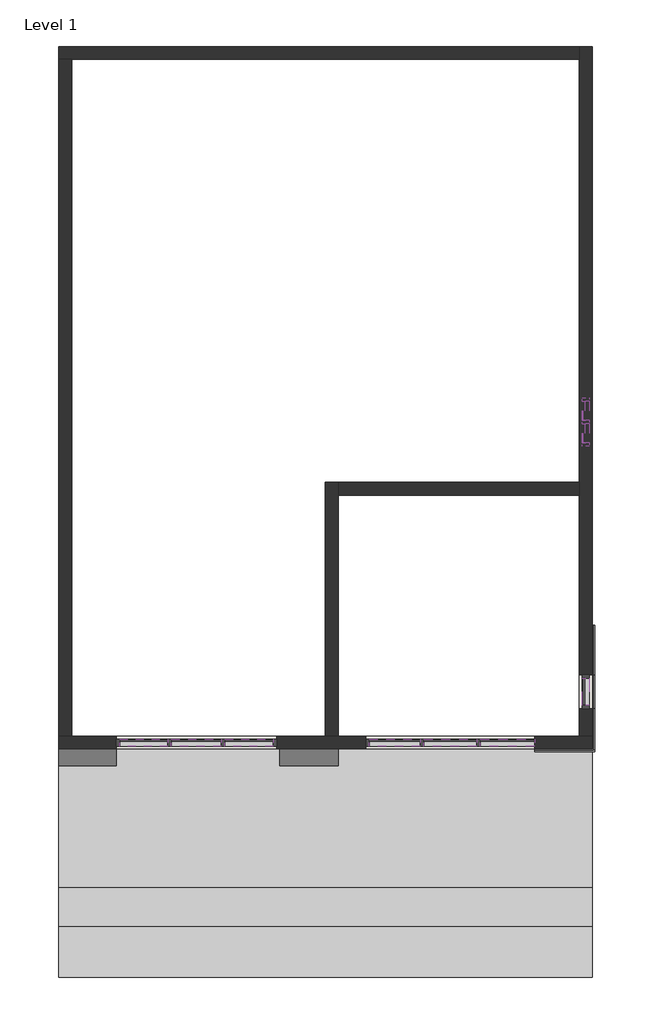
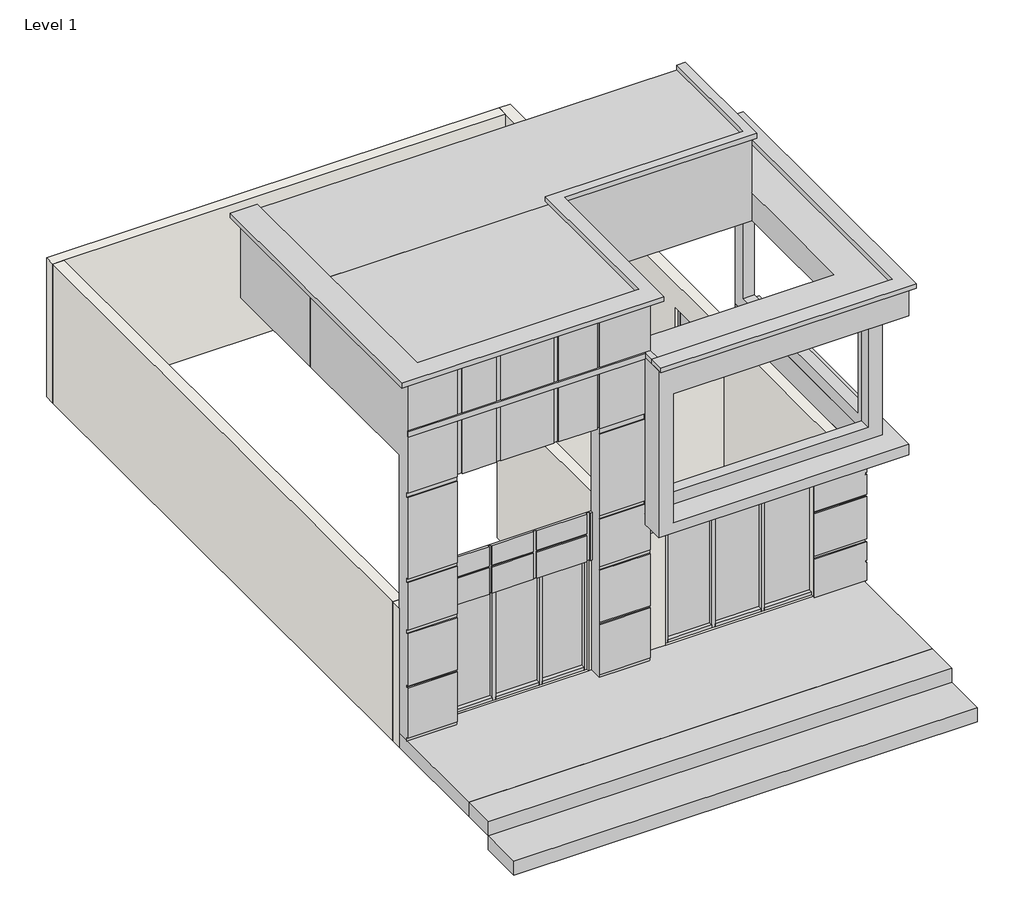
# One storey: 30 members, 9 plates, 6 walls, 3 proxies.
"""IFC4 building model written with IfcOpenShell, lengths in millimetres."""

from ifc_helpers import new_model, si_unit, origin, origin_with_axes, place, context, project, spatial, polyline, outline, extrude, faceted_brep, transform, mapped, element, save
from components import generic_models_1_generic_models_1_1e977ea9, generic_models_2_generic_models_2_230f2d88, generic_models_3_generic_models_3_1ac72cdd, member_ff1b7d8f, member_86d06fe4, member_33aca711, member_194e59d8, member_ff82125d, member_f5f6c3fe, member_be01e521, member_42d69148, member_024c663a, member_b7368e82, member_23836875, member_40a3ee5d, member_bb4f9a93, member_6db20980, system_panel_glazed_668e0709, system_panel_glazed_5062b81b, system_panel_glazed_581c84aa, system_panel_glazed_4d5331aa, system_panel_glazed_12377b85, system_panel_glazed_85e9b79d, system_panel_glazed_44434818

model = new_model("IFC4")

# Units and contexts
model_context = context("Model", 3, world=origin())
ifc_project = project(units=[si_unit("LENGTHUNIT", "METRE", prefix="MILLI")], contexts=[model_context])

# Site, building, storey
site = spatial("IfcSite", under=ifc_project)
building = spatial("IfcBuilding", under=site)
storey = spatial("IfcBuildingStorey", under=building, Name="Level 1", Elevation=0.0)

# Proxies
placement = place(None, origin())
generic_models_1_generic_models_1_shape = generic_models_1_generic_models_1_1e977ea9(model_context)
element("IfcBuildingElementProxy", 1, Name="Generic Models 1 : Generic Models 1", ObjectType="Generic Models 1 : Generic Models 1", at=placement, inside=storey, context=model_context, shape_type="MappedRepresentation", body=[
    mapped(generic_models_1_generic_models_1_shape, transform((0.0, 0.0, 0.0), x_axis=(1.0, 0.0, 0.0), y_axis=(0.0, 1.0, 0.0), z_axis=(0.0, 0.0, 1.0))),
])
generic_models_2_generic_models_2_shape = generic_models_2_generic_models_2_230f2d88(model_context)
element("IfcBuildingElementProxy", 2, Name="Generic Models 2 : Generic Models 2", ObjectType="Generic Models 2 : Generic Models 2", at=placement, inside=storey, context=model_context, shape_type="MappedRepresentation", body=[
    mapped(generic_models_2_generic_models_2_shape, transform((0.0, 0.0, 0.0), x_axis=(1.0, 0.0, 0.0), y_axis=(0.0, 1.0, 0.0), z_axis=(0.0, 0.0, 1.0))),
])
generic_models_3_generic_models_3_shape = generic_models_3_generic_models_3_1ac72cdd(model_context)
element("IfcBuildingElementProxy", 3, Name="Generic Models 3 : Generic Models 3", ObjectType="Generic Models 3 : Generic Models 3", at=placement, inside=storey, context=model_context, shape_type="MappedRepresentation", body=[
    mapped(generic_models_3_generic_models_3_shape, transform((0.0, 0.0, 0.0), x_axis=(1.0, 0.0, 0.0), y_axis=(0.0, 1.0, 0.0), z_axis=(0.0, 0.0, 1.0))),
])

# Members
member_shape = member_ff1b7d8f(model_context)
element("IfcMember", 4, ObjectType="Rectangular Mullion : 2.5\" x 5\" rectangular", at=placement, inside=storey, context=model_context, shape_type="MappedRepresentation", body=[
    mapped(member_shape, transform((-5727.4530968, -7048.658307, 1217.4178641), x_axis=(0.0, 0.0, -1.0), y_axis=(1.0, 0.0, 0.0), z_axis=(0.0, -1.0, 0.0))),
])
element("IfcMember", 5, ObjectType="Rectangular Mullion : 2.5\" x 5\" rectangular", at=placement, inside=storey, context=model_context, shape_type="MappedRepresentation", body=[
    mapped(member_shape, transform((-5727.4530968, -7455.058307, 1217.4178641), x_axis=(0.0, 0.0, -1.0), y_axis=(1.0, 0.0, 0.0), z_axis=(0.0, -1.0, 0.0))),
])
member_2_shape = member_86d06fe4(model_context)
element("IfcMember", 6, ObjectType="Rectangular Mullion : 2.5\" x 5\" rectangular", at=placement, inside=storey, context=model_context, shape_type="MappedRepresentation", body=[
    mapped(member_2_shape, transform((-5727.4530968, -12179.458307, 744.9879539), x_axis=(0.0, 0.0, -1.0), y_axis=(1.0, 0.0, 0.0), z_axis=(0.0, -1.0, 0.0))),
])
element("IfcMember", 7, ObjectType="Rectangular Mullion : 2.5\" x 5\" rectangular", at=placement, inside=storey, context=model_context, shape_type="MappedRepresentation", body=[
    mapped(member_2_shape, transform((-5727.4530968, -11696.858307, 2630.7756431), x_axis=(0.0, 0.0, 1.0), y_axis=(1.0, 0.0, 0.0), z_axis=(0.0, 1.0, 0.0))),
])
member_3_shape = member_33aca711(model_context)
element("IfcMember", 8, ObjectType="Rectangular Mullion : 2.5\" x 5\" rectangular", at=placement, inside=storey, context=model_context, shape_type="MappedRepresentation", body=[
    mapped(member_3_shape, transform((-5727.4530968, -11633.358307, 744.9879539), x_axis=(0.0, 1.0, 0.0), y_axis=(1.0, 0.0, 0.0), z_axis=(0.0, 0.0, -1.0))),
])
element("IfcMember", 9, ObjectType="Rectangular Mullion : 2.5\" x 5\" rectangular", at=placement, inside=storey, context=model_context, shape_type="MappedRepresentation", body=[
    mapped(member_3_shape, transform((-5727.4530968, -12242.958307, 2630.7756431), x_axis=(0.0, -1.0, 0.0), y_axis=(1.0, 0.0, 0.0), z_axis=(0.0, 0.0, 1.0))),
])
member_4_shape = member_194e59d8(model_context)
element("IfcMember", 10, ObjectType="Rectangular Mullion : 2.5\" x 5\" rectangular", at=placement, inside=storey, context=model_context, shape_type="MappedRepresentation", body=[
    mapped(member_4_shape, transform((-7689.6030968, -12852.558307, 2843.4388159), x_axis=(0.0, 0.0, 1.0), y_axis=(0.0, -1.0, 0.0), z_axis=(1.0, 0.0, 0.0))),
])
member_5_shape = member_ff82125d(model_context)
element("IfcMember", 11, ObjectType="Rectangular Mullion : 2.5\" x 5\" rectangular", at=placement, inside=storey, context=model_context, shape_type="MappedRepresentation", body=[
    mapped(member_5_shape, transform((-8705.6030968, -12852.558307, 2843.4388159), x_axis=(0.0, 0.0, 1.0), y_axis=(0.0, -1.0, 0.0), z_axis=(1.0, 0.0, 0.0))),
])
member_6_shape = member_f5f6c3fe(model_context)
element("IfcMember", 12, ObjectType="Rectangular Mullion : 2.5\" x 5\" rectangular", at=placement, inside=storey, context=model_context, shape_type="MappedRepresentation", body=[
    mapped(member_6_shape, transform((-6641.8530968, -12852.558307, 2843.4388159), x_axis=(0.0, 0.0, 1.0), y_axis=(0.0, -1.0, 0.0), z_axis=(1.0, 0.0, 0.0))),
])
member_7_shape = member_be01e521(model_context)
element("IfcMember", 13, ObjectType="Rectangular Mullion : 2.5\" x 5\" rectangular", at=placement, inside=storey, context=model_context, shape_type="MappedRepresentation", body=[
    mapped(member_7_shape, transform((-8673.8530968, -12852.558307, 304.8), x_axis=(1.0, 0.0, 0.0), y_axis=(0.0, -1.0, 0.0), z_axis=(0.0, 0.0, -1.0))),
])
element("IfcMember", 14, ObjectType="Rectangular Mullion : 2.5\" x 5\" rectangular", at=placement, inside=storey, context=model_context, shape_type="MappedRepresentation", body=[
    mapped(member_7_shape, transform((-7657.8530968, -12852.558307, 304.8), x_axis=(1.0, 0.0, 0.0), y_axis=(0.0, -1.0, 0.0), z_axis=(0.0, 0.0, -1.0))),
])
element("IfcMember", 15, ObjectType="Rectangular Mullion : 2.5\" x 5\" rectangular", at=placement, inside=storey, context=model_context, shape_type="MappedRepresentation", body=[
    mapped(member_6_shape, transform((-7626.1030968, -12852.558307, 304.8), x_axis=(0.0, 0.0, -1.0), y_axis=(0.0, -1.0, 0.0), z_axis=(-1.0, 0.0, 0.0))),
])
element("IfcMember", 16, ObjectType="Rectangular Mullion : 2.5\" x 5\" rectangular", at=placement, inside=storey, context=model_context, shape_type="MappedRepresentation", body=[
    mapped(member_4_shape, transform((-8642.1030968, -12852.558307, 304.8), x_axis=(0.0, 0.0, -1.0), y_axis=(0.0, -1.0, 0.0), z_axis=(-1.0, 0.0, 0.0))),
])
element("IfcMember", 17, ObjectType="Rectangular Mullion : 2.5\" x 5\" rectangular", at=placement, inside=storey, context=model_context, shape_type="MappedRepresentation", body=[
    mapped(member_5_shape, transform((-9626.3530968, -12852.558307, 304.8), x_axis=(0.0, 0.0, -1.0), y_axis=(0.0, -1.0, 0.0), z_axis=(-1.0, 0.0, 0.0))),
])
member_8_shape = member_42d69148(model_context)
element("IfcMember", 18, ObjectType="Rectangular Mullion : 2.5\" x 5\" rectangular", at=placement, inside=storey, context=model_context, shape_type="MappedRepresentation", body=[
    mapped(member_8_shape, transform((-9689.8530968, -12852.558307, 2843.4388159), x_axis=(-1.0, 0.0, 0.0), y_axis=(0.0, -1.0, 0.0), z_axis=(0.0, 0.0, 1.0))),
])
member_9_shape = member_024c663a(model_context)
element("IfcMember", 19, ObjectType="Rectangular Mullion : 2.5\" x 5\" rectangular", at=placement, inside=storey, context=model_context, shape_type="MappedRepresentation", body=[
    mapped(member_9_shape, transform((-13252.2030968, -12852.558307, 2744.8217298), x_axis=(0.0, 0.0, 1.0), y_axis=(0.0, -1.0, 0.0), z_axis=(1.0, 0.0, 0.0))),
])
element("IfcMember", 20, ObjectType="Rectangular Mullion : 2.5\" x 5\" rectangular", at=placement, inside=storey, context=model_context, shape_type="MappedRepresentation", body=[
    mapped(member_9_shape, transform((-11353.5530968, -12852.558307, 2744.8217298), x_axis=(0.0, 0.0, 1.0), y_axis=(0.0, -1.0, 0.0), z_axis=(1.0, 0.0, 0.0))),
])
member_10_shape = member_b7368e82(model_context)
element("IfcMember", 21, ObjectType="Rectangular Mullion : 2.5\" x 5\" rectangular", at=placement, inside=storey, context=model_context, shape_type="MappedRepresentation", body=[
    mapped(member_10_shape, transform((-12287.0030968, -12852.558307, 2744.8217298), x_axis=(0.0, 0.0, 1.0), y_axis=(0.0, -1.0, 0.0), z_axis=(1.0, 0.0, 0.0))),
])
member_11_shape = member_23836875(model_context)
element("IfcMember", 22, ObjectType="Rectangular Mullion : 2.5\" x 5\" rectangular", at=placement, inside=storey, context=model_context, shape_type="MappedRepresentation", body=[
    mapped(member_11_shape, transform((-13220.4530968, -12852.558307, 304.8), x_axis=(1.0, 0.0, 0.0), y_axis=(0.0, -1.0, 0.0), z_axis=(0.0, 0.0, -1.0))),
])
element("IfcMember", 23, ObjectType="Rectangular Mullion : 2.5\" x 5\" rectangular", at=placement, inside=storey, context=model_context, shape_type="MappedRepresentation", body=[
    mapped(member_11_shape, transform((-12255.2530968, -12852.558307, 304.8), x_axis=(1.0, 0.0, 0.0), y_axis=(0.0, -1.0, 0.0), z_axis=(0.0, 0.0, -1.0))),
])
element("IfcMember", 24, ObjectType="Rectangular Mullion : 2.5\" x 5\" rectangular", at=placement, inside=storey, context=model_context, shape_type="MappedRepresentation", body=[
    mapped(member_9_shape, transform((-12223.5030968, -12852.558307, 304.8), x_axis=(0.0, 0.0, -1.0), y_axis=(0.0, -1.0, 0.0), z_axis=(-1.0, 0.0, 0.0))),
])
element("IfcMember", 25, ObjectType="Rectangular Mullion : 2.5\" x 5\" rectangular", at=placement, inside=storey, context=model_context, shape_type="MappedRepresentation", body=[
    mapped(member_9_shape, transform((-14122.1530968, -12852.558307, 304.8), x_axis=(0.0, 0.0, -1.0), y_axis=(0.0, -1.0, 0.0), z_axis=(-1.0, 0.0, 0.0))),
])
element("IfcMember", 26, ObjectType="Rectangular Mullion : 2.5\" x 5\" rectangular", at=placement, inside=storey, context=model_context, shape_type="MappedRepresentation", body=[
    mapped(member_10_shape, transform((-13188.7030968, -12852.558307, 304.8), x_axis=(0.0, 0.0, -1.0), y_axis=(0.0, -1.0, 0.0), z_axis=(-1.0, 0.0, 0.0))),
])
member_12_shape = member_40a3ee5d(model_context)
element("IfcMember", 27, ObjectType="Rectangular Mullion : 2.5\" x 5\" rectangular", at=placement, inside=storey, context=model_context, shape_type="MappedRepresentation", body=[
    mapped(member_12_shape, transform((-14185.6530968, -12852.558307, 2744.8217298), x_axis=(-1.0, 0.0, 0.0), y_axis=(0.0, -1.0, 0.0), z_axis=(0.0, 0.0, 1.0))),
])
element("IfcMember", 28, ObjectType="Rectangular Mullion : 2.5\" x 5\" rectangular", at=placement, inside=storey, context=model_context, shape_type="MappedRepresentation", body=[
    mapped(member_12_shape, transform((-11290.0530968, -12852.558307, 304.8), x_axis=(1.0, 0.0, 0.0), y_axis=(0.0, -1.0, 0.0), z_axis=(0.0, 0.0, -1.0))),
])
element("IfcMember", 29, ObjectType="Rectangular Mullion : 2.5\" x 5\" rectangular", at=placement, inside=storey, context=model_context, shape_type="MappedRepresentation", body=[
    mapped(member_shape, transform((-5727.4530968, -7112.158307, 2505.4473458), x_axis=(0.0, 0.0, 1.0), y_axis=(1.0, 0.0, 0.0), z_axis=(0.0, 1.0, 0.0))),
])
element("IfcMember", 30, ObjectType="Rectangular Mullion : 2.5\" x 5\" rectangular", at=placement, inside=storey, context=model_context, shape_type="MappedRepresentation", body=[
    mapped(member_shape, transform((-5727.4530968, -6705.758307, 2505.4473458), x_axis=(0.0, 0.0, 1.0), y_axis=(1.0, 0.0, 0.0), z_axis=(0.0, 1.0, 0.0))),
])
member_13_shape = member_bb4f9a93(model_context)
element("IfcMember", 31, ObjectType="Rectangular Mullion : 2.5\" x 5\" rectangular", at=placement, inside=storey, context=model_context, shape_type="MappedRepresentation", body=[
    mapped(member_13_shape, transform((-5727.4530968, -7080.408307, 1217.4178641), x_axis=(0.0, 1.0, 0.0), y_axis=(1.0, 0.0, 0.0), z_axis=(0.0, 0.0, -1.0))),
])
member_14_shape = member_6db20980(model_context)
element("IfcMember", 32, ObjectType="Rectangular Mullion : 2.5\" x 5\" rectangular", at=placement, inside=storey, context=model_context, shape_type="MappedRepresentation", body=[
    mapped(member_14_shape, transform((-5727.4530968, -7518.558307, 2505.4473458), x_axis=(0.0, -1.0, 0.0), y_axis=(1.0, 0.0, 0.0), z_axis=(0.0, 0.0, 1.0))),
])
element("IfcMember", 33, ObjectType="Rectangular Mullion : 2.5\" x 5\" rectangular", at=placement, inside=storey, context=model_context, shape_type="MappedRepresentation", body=[
    mapped(member_14_shape, transform((-5727.4530968, -6642.258307, 1217.4178641), x_axis=(0.0, 1.0, 0.0), y_axis=(1.0, 0.0, 0.0), z_axis=(0.0, 0.0, -1.0))),
])

# Plates
system_panel_glazed_shape = system_panel_glazed_668e0709(model_context)
element("IfcPlate", 34, ObjectType="System Panel : Glazed", at=placement, inside=storey, context=model_context, shape_type="MappedRepresentation", body=[
    mapped(system_panel_glazed_shape, transform((-5727.4530968, -11938.158307, 808.4879539), x_axis=(0.0, 1.0, 0.0), y_axis=(-1.0, 0.0, 0.0), z_axis=(0.0, 0.0, 1.0))),
])
system_panel_glazed_2_shape = system_panel_glazed_5062b81b(model_context)
element("IfcPlate", 35, ObjectType="System Panel : Glazed", at=placement, inside=storey, context=model_context, shape_type="MappedRepresentation", body=[
    mapped(system_panel_glazed_2_shape, transform((-9165.9780968, -12852.558307, 368.3), x_axis=(1.0, 0.0, 0.0), y_axis=(0.0, 1.0, 0.0), z_axis=(0.0, 0.0, 1.0))),
])
system_panel_glazed_3_shape = system_panel_glazed_581c84aa(model_context)
element("IfcPlate", 36, ObjectType="System Panel : Glazed", at=placement, inside=storey, context=model_context, shape_type="MappedRepresentation", body=[
    mapped(system_panel_glazed_3_shape, transform((-8165.8530968, -12852.558307, 368.3), x_axis=(1.0, 0.0, 0.0), y_axis=(0.0, 1.0, 0.0), z_axis=(0.0, 0.0, 1.0))),
])
system_panel_glazed_4_shape = system_panel_glazed_4d5331aa(model_context)
element("IfcPlate", 37, ObjectType="System Panel : Glazed", at=placement, inside=storey, context=model_context, shape_type="MappedRepresentation", body=[
    mapped(system_panel_glazed_4_shape, transform((-7133.9780968, -12852.558307, 368.3), x_axis=(1.0, 0.0, 0.0), y_axis=(0.0, 1.0, 0.0), z_axis=(0.0, 0.0, 1.0))),
])
system_panel_glazed_5_shape = system_panel_glazed_12377b85(model_context)
element("IfcPlate", 38, ObjectType="System Panel : Glazed", at=placement, inside=storey, context=model_context, shape_type="MappedRepresentation", body=[
    mapped(system_panel_glazed_5_shape, transform((-13687.1780968, -12852.558307, 368.3), x_axis=(1.0, 0.0, 0.0), y_axis=(0.0, 1.0, 0.0), z_axis=(0.0, 0.0, 1.0))),
])
element("IfcPlate", 39, ObjectType="System Panel : Glazed", at=placement, inside=storey, context=model_context, shape_type="MappedRepresentation", body=[
    mapped(system_panel_glazed_5_shape, transform((-11788.5280968, -12852.558307, 368.3), x_axis=(1.0, 0.0, 0.0), y_axis=(0.0, 1.0, 0.0), z_axis=(0.0, 0.0, 1.0))),
])
system_panel_glazed_6_shape = system_panel_glazed_85e9b79d(model_context)
element("IfcPlate", 40, ObjectType="System Panel : Glazed", at=placement, inside=storey, context=model_context, shape_type="MappedRepresentation", body=[
    mapped(system_panel_glazed_6_shape, transform((-12737.8530968, -12852.558307, 368.3), x_axis=(1.0, 0.0, 0.0), y_axis=(0.0, 1.0, 0.0), z_axis=(0.0, 0.0, 1.0))),
])
system_panel_glazed_7_shape = system_panel_glazed_44434818(model_context)
element("IfcPlate", 41, ObjectType="System Panel : Glazed", at=placement, inside=storey, context=model_context, shape_type="MappedRepresentation", body=[
    mapped(system_panel_glazed_7_shape, transform((-5727.4530968, -7283.608307, 1280.9178641), x_axis=(0.0, 1.0, 0.0), y_axis=(-1.0, 0.0, 0.0), z_axis=(0.0, 0.0, 1.0))),
])
element("IfcPlate", 42, ObjectType="System Panel : Glazed", at=placement, inside=storey, context=model_context, shape_type="MappedRepresentation", body=[
    mapped(system_panel_glazed_7_shape, transform((-5727.4530968, -6877.208307, 1280.9178641), x_axis=(0.0, 1.0, 0.0), y_axis=(-1.0, 0.0, 0.0), z_axis=(0.0, 0.0, 1.0))),
])

# Walls
element("IfcWall", 43, ObjectType="9\"", at=placement, inside=storey, context=model_context, shape_type="Brep", body=[
    faceted_brep([(-15214.3530968, -12966.858307, 0.0), (-5613.1530968, -12966.858307, 0.0), (-5613.1530968, -12966.858307, 3048.0), (-15214.3530968, -12966.858307, 3048.0), (-14185.6530968, -12966.858307, 304.8), (-14185.6530968, -12966.858307, 2744.8217298), (-11290.0530968, -12966.858307, 2744.8217298), (-11290.0530968, -12966.858307, 304.8), (-9689.8530968, -12966.858307, 304.8), (-9689.8530968, -12966.858307, 2843.4388159), (-6641.8530968, -12966.858307, 2843.4388159), (-6641.8530968, -12966.858307, 304.8), (-5613.1530968, -12738.258307, 0.0), (-5841.7530968, -12738.258307, 0.0), (-10185.1530968, -12738.258307, 0.0), (-10413.7530968, -12738.258307, 0.0), (-14985.7530968, -12738.258307, 0.0), (-15214.3530968, -12738.258307, 0.0), (-15214.3530968, -12738.258307, 3048.0), (-14985.7530968, -12738.258307, 3048.0), (-10413.7530968, -12738.258307, 3048.0), (-10185.1530968, -12738.258307, 3048.0), (-5841.7530968, -12738.258307, 3048.0), (-5613.1530968, -12738.258307, 3048.0), (-14185.6530968, -12738.258307, 2744.8217298), (-14185.6530968, -12738.258307, 304.8), (-11290.0530968, -12738.258307, 304.8), (-11290.0530968, -12738.258307, 2744.8217298), (-9689.8530968, -12738.258307, 2843.4388159), (-9689.8530968, -12738.258307, 304.8), (-6641.8530968, -12738.258307, 304.8), (-6641.8530968, -12738.258307, 2843.4388159)], [[[0, 1, 2, 3], [4, 5, 6, 7], [8, 9, 10, 11]], [[12, 13, 14, 15, 16, 17, 18, 19, 20, 21, 22, 23], [24, 25, 26, 27], [28, 29, 30, 31]], [[1, 0, 17, 16, 15, 14, 13, 12]], [[3, 2, 23, 22, 21, 20, 19, 18]], [[2, 1, 12, 23]], [[0, 3, 18, 17]], [[24, 5, 4, 25]], [[5, 24, 27, 6]], [[6, 27, 26, 7]], [[25, 4, 7, 26]], [[8, 29, 28, 9]], [[9, 28, 31, 10]], [[10, 31, 30, 11]], [[29, 8, 11, 30]]]),
])
element("IfcWall", 44, ObjectType="9\"", at=placement, inside=storey, context=model_context, shape_type="Brep", body=[
    faceted_brep([(-5613.1530968, -12738.258307, 0.0), (-5613.1530968, -317.658307, 0.0), (-5613.1530968, -317.658307, 3048.0), (-5613.1530968, -12738.258307, 3048.0), (-5613.1530968, -12242.958307, 744.9879539), (-5613.1530968, -12242.958307, 2630.7756431), (-5613.1530968, -11633.358307, 2630.7756431), (-5613.1530968, -11633.358307, 744.9879539), (-5613.1530968, -7518.558307, 1217.4178641), (-5613.1530968, -7518.558307, 2505.4473458), (-5613.1530968, -6642.258307, 2505.4473458), (-5613.1530968, -6642.258307, 1217.4178641), (-5841.7530968, -317.658307, 0.0), (-5841.7530968, -546.258307, 0.0), (-5841.7530968, -8166.258307, 0.0), (-5841.7530968, -8394.858307, 0.0), (-5841.7530968, -12738.258307, 0.0), (-5841.7530968, -12738.258307, 3048.0), (-5841.7530968, -8394.858307, 3048.0), (-5841.7530968, -8166.258307, 3048.0), (-5841.7530968, -546.258307, 3048.0), (-5841.7530968, -317.658307, 3048.0), (-5841.7530968, -12242.958307, 2630.7756431), (-5841.7530968, -12242.958307, 744.9879539), (-5841.7530968, -11633.358307, 744.9879539), (-5841.7530968, -11633.358307, 2630.7756431), (-5841.7530968, -7518.558307, 2505.4473458), (-5841.7530968, -7518.558307, 1217.4178641), (-5841.7530968, -6642.258307, 1217.4178641), (-5841.7530968, -6642.258307, 2505.4473458)], [[[0, 1, 2, 3], [4, 5, 6, 7], [8, 9, 10, 11]], [[12, 13, 14, 15, 16, 17, 18, 19, 20, 21], [22, 23, 24, 25], [26, 27, 28, 29]], [[1, 0, 16, 15, 14, 13, 12]], [[3, 2, 21, 20, 19, 18, 17]], [[0, 3, 17, 16]], [[2, 1, 12, 21]], [[22, 5, 4, 23]], [[5, 22, 25, 6]], [[6, 25, 24, 7]], [[23, 4, 7, 24]], [[8, 27, 26, 9]], [[9, 26, 29, 10]], [[10, 29, 28, 11]], [[27, 8, 11, 28]]]),
])
element("IfcWall", 45, ObjectType="9\"", at=placement, inside=storey, context=model_context, shape_type="Brep", body=[
    faceted_brep([(-5841.7530968, -317.658307, 0.0), (-15214.3530968, -317.658307, 0.0), (-15214.3530968, -317.658307, 3048.0), (-5841.7530968, -317.658307, 3048.0), (-5841.7530968, -546.258307, 0.0), (-5841.7530968, -546.258307, 3048.0), (-14985.7530968, -546.258307, 3048.0), (-15214.3530968, -546.258307, 3048.0), (-15214.3530968, -546.258307, 0.0), (-14985.7530968, -546.258307, 0.0)], [[[0, 1, 2, 3]], [[4, 5, 6, 7, 8, 9]], [[1, 0, 4, 9, 8]], [[3, 2, 7, 6, 5]], [[0, 3, 5, 4]], [[2, 1, 8, 7]]]),
])
element("IfcWall", 46, ObjectType="9\"", at=placement, inside=storey, context=model_context, shape_type="SweptSolid", body=[
    extrude(outline(polyline([(-15214.3530968, -12738.258307), (-15214.3530968, -546.258307), (-14985.7530968, -546.258307), (-14985.7530968, -12738.258307), (-15214.3530968, -12738.258307)])), origin_with_axes(), (0.0, 0.0, 1.0), 3048.0),
])
element("IfcWall", 47, ObjectType="9\"", at=placement, inside=storey, context=model_context, shape_type="Brep", body=[
    faceted_brep([(-10185.1530968, -12738.258307, 0.0), (-10185.1530968, -8394.858307, 0.0), (-10185.1530968, -8166.258307, 0.0), (-10185.1530968, -8166.258307, 3048.0), (-10185.1530968, -8394.858307, 3048.0), (-10185.1530968, -12738.258307, 3048.0), (-10413.7530968, -12738.258307, 0.0), (-10413.7530968, -12738.258307, 3048.0), (-10413.7530968, -8166.258307, 3048.0), (-10413.7530968, -8166.258307, 0.0)], [[[0, 1, 2, 3, 4, 5]], [[6, 7, 8, 9]], [[2, 1, 0, 6, 9]], [[5, 4, 3, 8, 7]], [[0, 5, 7, 6]], [[3, 2, 9, 8]]]),
])
element("IfcWall", 48, ObjectType="9\"", at=placement, inside=storey, context=model_context, shape_type="SweptSolid", body=[
    extrude(outline(polyline([(-5841.7530968, -8394.858307), (-10185.1530968, -8394.858307), (-10185.1530968, -8166.258307), (-5841.7530968, -8166.258307), (-5841.7530968, -8394.858307)])), origin_with_axes(), (0.0, 0.0, 1.0), 3048.0),
])

save(model, "model.ifc")

# Revit data of these elements
# Type "Rectangular Mullion : 2.5\" x 5\" rectangular"
#   built-in parameter 1007304 = 0.416667 (stored number, unit not read)
#   built-in parameter 1007301 = 0.104167 (stored number, unit not read)
#   built-in parameter 1007300 = 0.104167 (stored number, unit not read)
# Type "System Panel : Glazed"
#   Construction Type Id = "GSP4R"
#   Analytic Construction = "1/8 in Pilkington single glazing"
#   Visual Light Transmittance = 0.9
#   Solar Heat Gain Coefficient = 0.86
#   Heat Transfer Coefficient (U) = 1.18115 BTU/(h·ft²·°F)
#   Define Thermal Properties by = 1
# Type "9\""
#   Assembly Code = "B2010"
#   Layers, outside or top first: 0' - 9" no material (function 1)
# Element 1 (IfcBuildingElementProxy, "Generic Models 1 : Generic Models 1")
#   Phase Created = New Construction
# Element 2 (IfcBuildingElementProxy, "Generic Models 2 : Generic Models 2")
#   Phase Created = New Construction
# Element 3 (IfcBuildingElementProxy, "Generic Models 3 : Generic Models 3")
#   Phase Created = New Construction
#   Materials on its faces: "Structure, Wood Joist/Rafter Layer, Batt Insulation"
# Elements 4, 5, 6, 7, 8, 9, 10, 11, 12, 13, 14, 15, 16, 17, 18, 19, 20, 21, 22, 23, 24, 25, 26, 27, 28, 29, 30, 31, 32, 33 (IfcMember, "Rectangular Mullion : 2.5\" x 5\" rectangular")
#   Phase Created = New Construction
#   Materials on its faces: "Aluminum"
# Elements 34, 35, 36, 37, 38, 39, 40, 41, 42 (IfcPlate, "System Panel : Glazed")
#   Phase Created = New Construction
#   Materials on its faces: "Glass"
# Elements 43, 44, 45, 46, 47, 48 (IfcWall, "9\"")
#   Top Offset = 0' - 0"
#   Base Offset = 0' - 0"
#   Unconnected Height = 10' - 0"
#   wall height = 10' - 0"
#   Phase Created = New Construction
#   Base Constraint = Level 1
#   Materials on its faces: "Default Wall"
# Materials
#   "Structure, Wood Joist/Rafter Layer, Batt Insulation": class "Wood", colour RGB 127 127 127, transparency 0, Description = "Wood framing, insulated", Cost = 0
#   "Aluminum": class "Metal", colour RGB 247 247 247, transparency 0, Description = "Aluminum 6061", Cost = 0
#   "Glass": class "Glass", colour RGB 0 128 192, transparency 0.75, Description = "Soda Lime Glass", Cost = 0
#   "Default Wall": colour RGB 128 128 128, transparency 0, Cost = 0
